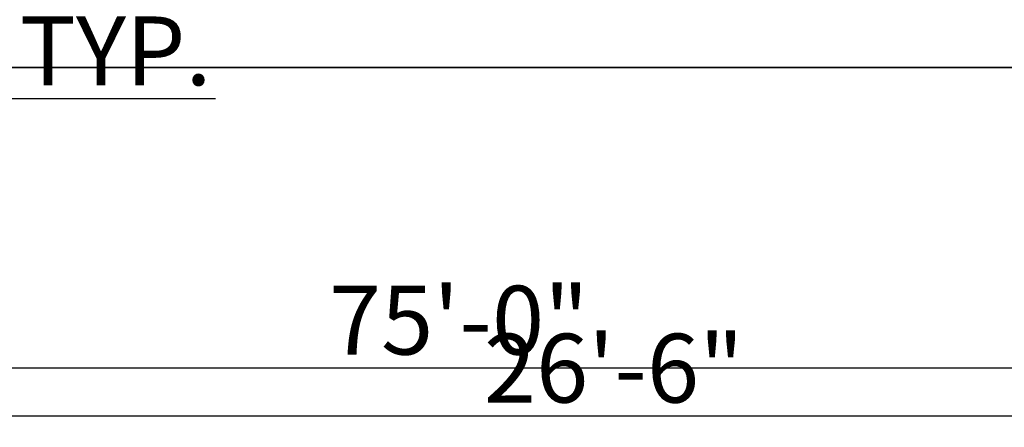
# Model space of a CAD drawing. Units: inches. Extents: x 2083 to 3317, y 1141 to 2115.
# Tile 106 of 256: x 2600 to 2772, y 1201 to 1272. Entities that reach past the tile are written whole.
import ezdxf

# ---------------------------------------------------------------- set-up
doc = ezdxf.new("R2010")
doc.units = ezdxf.units.IN
doc.layers.add('A-ANNO-DIMS', color=2, linetype='Continuous', lineweight=18)
doc.layers.add('A-WALL', color=7, linetype='Continuous', lineweight=35)
doc.layers.add('A-WALL-PATT', color=251, linetype='Continuous', lineweight=13, true_color=0x636466)
doc.styles.get("Standard").update_dxf_attribs({"font": 'arial.ttf'})
doc.dimstyles.new('ISO-25', dxfattribs={"dimtxt": 12, "dimasz": 12, "dimexe": 1.25, "dimexo": 0.625, "dimtad": 1, "dimlunit": 3, "dimtxsty": 'Standard', "dimcen": 2.5, "dimadec": 0, "dimazin": 0, "dimtfac": 1, "dimtmove": 0, "dimatfit": 3, "dimfxl": 1, "dimarcsym": 0})

# ---------------------------------------------------------------- blocks, each defined once
blk = doc.blocks.new('*D11')
at = {"layer": 'A-ANNO-DIMS', "color": 0, "lineweight": -2, "transparency": 16777216}
for p, q in [((2544.96, 1262.64), (2544.96, 1201.28)), ((2862.96, 1262.64), (2862.96, 1201.28)), ((2556.96, 1202.53), (2850.96, 1202.53))]:
    blk.add_line(p, q, dxfattribs=at)
at = {"layer": 'A-ANNO-DIMS', "color": 0, "transparency": 16777216}
for points in [[(2556.96, 1204.53), (2556.96, 1200.53), (2544.96, 1202.53)], [(2850.96, 1204.53), (2850.96, 1200.53), (2862.96, 1202.53)]]:
    blk.add_solid(points, dxfattribs=at)
at = {"layer": 'Defpoints', "color": 0, "transparency": 16777216}
for p in [(2544.96, 1263.26), (2862.96, 1263.26), (2862.96, 1202.53)]:
    blk.add_point(p, dxfattribs=at)
at = {"layer": 'A-ANNO-DIMS', "color": 0, "transparency": 16777216, "insert": (2703.96, 1209.29), "char_height": 12, "attachment_point": 5}
blk.add_mtext('26\'-6"', dxfattribs=at)
blk = doc.blocks.new('*D25')
at = {"layer": 'A-ANNO-DIMS', "color": 0, "lineweight": -2, "transparency": 16777216}
for p, q in [((2511.96, 1271.64), (2511.96, 1256.61)), ((2535.96, 1271.64), (2535.96, 1256.61)), ((2499.96, 1257.86), (2487.96, 1257.86)), ((2511.96, 1257.86), (2535.96, 1257.86)), ((2547.96, 1257.86), (2634.56, 1257.86))]:
    blk.add_line(p, q, dxfattribs=at)
at = {"layer": 'A-ANNO-DIMS', "color": 0, "transparency": 16777216}
for points in [[(2499.96, 1259.86), (2499.96, 1255.86), (2511.96, 1257.86)], [(2547.96, 1259.86), (2547.96, 1255.86), (2535.96, 1257.86)]]:
    blk.add_solid(points, dxfattribs=at)
at = {"layer": 'Defpoints', "color": 0, "transparency": 16777216}
for p in [(2511.96, 1272.26), (2535.96, 1272.26), (2535.96, 1257.86)]:
    blk.add_point(p, dxfattribs=at)
at = {"layer": 'A-ANNO-DIMS', "color": 0, "transparency": 16777216, "insert": (2597.26, 1264.61), "char_height": 12, "attachment_point": 5}
blk.add_mtext('2\'-0" TYP.', dxfattribs=at)
blk = doc.blocks.new('*D34')
at = {"layer": 'A-ANNO-DIMS', "color": 0, "lineweight": -2, "transparency": 16777216}
for p, q in [((2226.96, 1262.64), (2226.96, 1209.66)), ((3126.96, 1262.64), (3126.96, 1209.66)), ((2238.96, 1210.91), (3114.96, 1210.91))]:
    blk.add_line(p, q, dxfattribs=at)
at = {"layer": 'A-ANNO-DIMS', "color": 0, "transparency": 16777216}
for points in [[(2238.96, 1212.91), (2238.96, 1208.91), (2226.96, 1210.91)], [(3114.96, 1212.91), (3114.96, 1208.91), (3126.96, 1210.91)]]:
    blk.add_solid(points, dxfattribs=at)
at = {"layer": 'Defpoints', "color": 0, "transparency": 16777216}
for p in [(2226.96, 1263.26), (3126.96, 1263.26), (3126.96, 1210.91)]:
    blk.add_point(p, dxfattribs=at)
at = {"layer": 'A-ANNO-DIMS', "color": 0, "transparency": 16777216, "insert": (2676.96, 1217.66), "char_height": 12, "attachment_point": 5}
blk.add_mtext('75\'-0"', dxfattribs=at)

msp = doc.modelspace()

# ---------------------------------------------------------------- hatches: boundary and pattern name
at = {"layer": 'A-WALL-PATT'}
h = msp.add_hatch(color=256, dxfattribs=at)
h.dxf.hatch_style = 1
h.paths.add_polyline_path([(3126.96, 2020.761), (2748.96, 2020.761), (2604.96, 2020.761), (2226.96, 2020.761), (2226.96, 1702.761), (2466.96, 1702.761), (2466.96, 1582.761), (2418.96, 1582.761), (2418.96, 1477.761), (2226.96, 1477.761), (2226.96, 1263.261), (2544.96, 1263.261), (2544.96, 1411.761), (2604.96, 1411.761), (2685.96, 1411.761), (2685.96, 1420.761), (2604.96, 1420.761), (2604.96, 1573.761), (2604.96, 1702.761), (2604.96, 2011.761), (2748.96, 2011.761), (2748.96, 1702.761), (2862.96, 1702.761), (2862.96, 1621.761), (2871.96, 1621.761), (2871.96, 1702.761), (2883.96, 1702.761), (2883.96, 1706.939, -0.0264593), (2883.96, 1711.761), (2757.96, 1711.761), (2757.96, 1807.761), (2787.96, 1807.761), (2787.96, 1812.261), (2757.96, 1812.261), (2757.96, 2011.761), (2877.96, 2011.761), (2877.96, 1812.261), (2847.96, 1812.261), (2847.96, 1807.761), (2889.836, 1807.761), (2889.836, 1812.261), (2882.46, 1812.261), (2882.46, 2011.761), (3117.96, 2011.761), (3117.96, 1812.261), (2937.836, 1812.261), (2937.836, 1807.761), (2995.71, 1807.761), (2995.71, 1796.118), (3000.21, 1796.118), (3000.21, 1807.761), (3117.96, 1807.761), (3117.96, 1711.761), (3000.21, 1711.761), (3000.21, 1760.118), (2998.573, 1760.118, -0.020711), (2995.71, 1760.118), (2995.71, 1711.761), (2931.96, 1711.761), (2931.96, 1702.761), (3126.96, 1702.761)])
h.paths.add_polyline_path([(2471.46, 2011.761), (2471.46, 1810.011), (2462.717, 1810.011), (2462.717, 1805.511), (2505.96, 1805.511), (2505.96, 1810.011), (2475.96, 1810.011), (2475.96, 2011.761), (2595.96, 2011.761), (2595.96, 1810.011), (2565.96, 1810.011), (2565.96, 1805.511), (2595.96, 1805.511), (2595.96, 1711.761), (2235.96, 1711.761), (2235.96, 1805.511), (2353.71, 1805.511), (2353.71, 1796.054), (2358.21, 1796.054), (2358.21, 1805.511), (2414.717, 1805.511), (2414.717, 1810.011), (2235.96, 1810.011), (2235.96, 2011.761)], flags=16)
h.paths.add_polyline_path([(2270.205, 1994.61), (2270.205, 1970.61), (2246.205, 1970.61), (2246.205, 1994.61)], flags=0)
edge = h.paths.add_edge_path(flags=0)
edge.add_ellipse((2332.027, 1899.798), major_axis=(-3.043, 3.043), ratio=0.1682525, start_angle=-161.33217, end_angle=-156.30711, ccw=False)
edge.add_ellipse((2333.082, 1898.744), major_axis=(-1.055, 1.055), ratio=0.4535321, start_angle=-123.37102, end_angle=-94.15911)
edge = h.paths.add_edge_path(flags=0)
edge.add_ellipse((2332.027, 1968.876), major_axis=(3.043, 3.043), ratio=0.1682525, start_angle=18.66783, end_angle=23.69289)
edge.add_spline(control_points=[(2332.926, 1970.691), (2332.227, 1970.336), (2330.894, 1969.659), (2328.413, 1970.932), (2327.204, 1967.749), (2324.71, 1969.956), (2322.533, 1967.012), (2320.013, 1971.296), (2317.68, 1968.158), (2316.041, 1967.102), (2315.427, 1966.81)], knot_values=[0, 0, 0, 0, 2.2670587, 4.3245589, 6.6855835, 8.8786411, 11.121502, 14.300359, 17.7552837, 19.732645, 19.732645, 19.732645, 19.732645], degree=3, periodic=0)
edge.add_ellipse((2332.027, 1968.876), major_axis=(3.043, 3.043), ratio=0.1682525, start_angle=18.66783, end_angle=23.69289, ccw=False)
edge.add_ellipse((2333.082, 1969.931), major_axis=(1.055, 1.055), ratio=0.4535321, start_angle=56.62898, end_angle=85.84089, ccw=False)
edge = h.paths.add_edge_path(flags=0)
edge.add_spline(control_points=[(2296.428, 1967.988), (2293.628, 1965.336), (2287.704, 1959.727), (2299.744, 1949.996), (2294.533, 1935.669), (2290.573, 1920.604), (2293.394, 1909.974), (2296.185, 1904.967)], knot_values=[0.0991853, 0.0991853, 0.0991853, 0.0991853, 0.3453009, 0.6198217, 0.9826526, 1.3860932, 1.8105546, 1.8105546, 1.8105546, 1.8105546], degree=3, periodic=0)
edge.add_spline(control_points=[(2296.185, 1904.967), (2297.384, 1902.619), (2298.001, 1901.949), (2298.553, 1901.468)], knot_values=[0.0062457, 0.0062457, 0.0062457, 0.0062457, 0.0554759, 0.0554759, 0.0554759, 0.0554759], degree=3, periodic=0)
edge.add_spline(control_points=[(2298.553, 1901.468), (2297.259, 1900.923), (2295.225, 1900.232), (2293.06, 1900.614), (2292.101, 1900.788), (2292.09, 1900.791)], knot_values=[0.3128349, 0.3128349, 0.3128349, 0.3128349, 0.4017797, 0.4749867, 0.4759027, 0.4759027, 0.4759027, 0.4759027], degree=3, periodic=0)
edge.add_arc((2292.794, 1904.664), 3.937, 215.4209, 259.69818, ccw=False)
edge.add_spline(control_points=[(2289.585, 1902.382), (2289.477, 1902.535), (2289.368, 1902.688), (2289.261, 1902.841)], knot_values=[0.1028719, 0.1028719, 0.1028719, 0.1028719, 0.1168958, 0.1168958, 0.1168958, 0.1168958], degree=3, periodic=0)
edge.add_spline(control_points=[(2289.261, 1902.841), (2288.687, 1902.55), (2287.64, 1902.02), (2285.881, 1901.874), (2283.853, 1901.504), (2281.72, 1899.711), (2278.467, 1899.493), (2276.157, 1901.883), (2272.259, 1899.804), (2267.778, 1901.843), (2262.244, 1900.184), (2257.415, 1901.782), (2254.318, 1900.726), (2253.178, 1900.337)], knot_values=[0, 0, 0, 0, 1.9079767, 3.4771759, 5.261074, 7.9728515, 11.6802485, 13.7179214, 16.9395917, 22.789562, 27.5025027, 33.5952153, 37.1456181, 37.1456181, 37.1456181, 37.1456181], degree=3, periodic=0)
edge.add_line((2253.178, 1900.337), (2250.244, 1902.841))
edge.add_line((2250.244, 1902.841), (2250.244, 1965.833))
edge.add_line((2250.244, 1965.833), (2253.178, 1968.337))
edge.add_spline(control_points=[(2253.178, 1968.337), (2254.318, 1967.948), (2257.415, 1966.892), (2262.244, 1968.49), (2267.778, 1966.831), (2271.527, 1968.537), (2273.876, 1967.828), (2274.207, 1967.728)], knot_values=[0, 0, 0, 0, 0.0901802, 0.2449351, 0.3646438, 0.5132331, 0.5378548, 0.5378548, 0.5378548, 0.5378548], degree=3, periodic=0)
edge.add_arc((2274.353, 1963.793), 3.937, 72.05113, 92.12795, ccw=False)
edge.add_arc((2281.297, 1985.23), 18.596, 252.05113, 288.56572)
edge.add_arc((2292.317, 1956.029), 12.646, 71.02679, 113.77822, ccw=False)
edge = h.paths.add_edge_path(flags=0)
edge.add_spline(control_points=[(2274.899, 1951.856), (2275.066, 1951.617), (2275.233, 1951.377), (2275.398, 1951.136)], knot_values=[1.4099157, 1.4099157, 1.4099157, 1.4099157, 1.4315903, 1.4315903, 1.4315903, 1.4315903], degree=3, periodic=0)
edge.add_spline(control_points=[(2275.398, 1951.136), (2275.792, 1950.562), (2276.179, 1949.984), (2276.546, 1949.397)], knot_values=[1.3582378, 1.3582378, 1.3582378, 1.3582378, 1.4099157, 1.4099157, 1.4099157, 1.4099157], degree=3, periodic=0)
edge.add_line((2276.546, 1949.397), (2277.437, 1947.862))
edge.add_spline(control_points=[(2277.437, 1947.862), (2276.304, 1945.673), (2274.64, 1942.427), (2274.632, 1938.094), (2272.799, 1930.852), (2274.356, 1943.897), (2275.948, 1947.923), (2276.546, 1949.397)], knot_values=[0.0056315, 0.0056315, 0.0056315, 0.0056315, 0.1860139, 0.2660015, 0.3570872, 0.5963902, 0.7397317, 0.7397317, 0.7397317, 0.7397317], degree=3, periodic=0)
edge.add_spline(control_points=[(2276.546, 1949.397), (2276.179, 1949.984), (2275.792, 1950.562), (2275.398, 1951.136)], knot_values=[1.3582378, 1.3582378, 1.3582378, 1.3582378, 1.4099157, 1.4099157, 1.4099157, 1.4099157], degree=3, periodic=0)
edge.add_spline(control_points=[(2275.398, 1951.136), (2274.943, 1950.08), (2274.208, 1948.025), (2273.935, 1944.851), (2272.469, 1937.627), (2273.466, 1945.696), (2274.701, 1951.059), (2274.899, 1951.856)], knot_values=[0.1043639, 0.1043639, 0.1043639, 0.1043639, 0.1896363, 0.2696239, 0.3607096, 0.6000126, 0.6446217, 0.6446217, 0.6446217, 0.6446217], degree=3, periodic=0)
h.paths.add_polyline_path([(2269.168, 1963.128, -0.3575267), (2268.171, 1960.976, -0.0925607), (2268.171, 1939.436, -0.3575267), (2269.168, 1937.285, -0.3575267), (2267.016, 1938.282, -0.1647847), (2254.686, 1938.282, -0.3575267), (2252.534, 1937.285, -0.3575267), (2253.531, 1939.436, -0.0925607), (2253.531, 1960.976, -0.3575267), (2252.534, 1963.128, -0.3575267), (2254.686, 1962.131, -0.1647847), (2267.016, 1962.131, -0.3575267)], flags=0)
h.paths.add_polyline_path([(2248.874, 1967.802), (2248.874, 1957.028), (2249.458, 1957.028), (2249.458, 1911.647), (2248.874, 1911.647), (2248.874, 1900.873), (2246.512, 1900.873, 0.1973271), (2244.15, 1902.457), (2244.15, 1966.218, 0.1973271), (2246.512, 1967.802)], flags=0)
h.paths.add_polyline_path([(2269.168, 1931.389, -0.3575267), (2268.171, 1929.238, -0.0925607), (2268.171, 1907.698, -0.3575267), (2269.168, 1905.547, -0.3575267), (2267.016, 1906.544, -0.1647847), (2254.686, 1906.544, -0.3575267), (2252.534, 1905.547, -0.3575267), (2253.531, 1907.698, -0.0925607), (2253.531, 1929.238, -0.3575267), (2252.534, 1931.389, -0.3575267), (2254.686, 1930.392, -0.1647847), (2267.016, 1930.392, -0.3575267)], flags=0)
edge = h.paths.add_edge_path(flags=0)
edge.add_spline(control_points=[(2276.197, 1906.724), (2276.168, 1909.029), (2276.114, 1913.372), (2270.598, 1924.925), (2273.905, 1919.013), (2275.922, 1916.262), (2275.475, 1912.402), (2277.258, 1910.381), (2276.696, 1908.225), (2276.646, 1906.813), (2276.618, 1906.008)], knot_values=[0, 0, 0, 0, 8.6102597, 16.2212739, 18.8430575, 23.8048978, 27.4408283, 29.3561016, 31.2034776, 33.6506866, 33.6506866, 33.6506866, 33.6506866], degree=3, periodic=0)
edge.add_spline(control_points=[(2276.618, 1906.008), (2276.623, 1905.624), (2276.498, 1904.629), (2275.442, 1903.855), (2274.937, 1903.08), (2274.859, 1902.841)], knot_values=[0.1564884, 0.1564884, 0.1564884, 0.1564884, 0.1843975, 0.2313765, 0.2505985, 0.2505985, 0.2505985, 0.2505985], degree=3, periodic=0)
edge.add_line((2274.859, 1902.841), (2276.506, 1902.841))
edge.add_spline(control_points=[(2276.506, 1902.841), (2276.788, 1903.085), (2277.665, 1904.125), (2278.25, 1904.341), (2277.654, 1908.527), (2278.156, 1906.228), (2278.1, 1905.286), (2278.847, 1904.069), (2277.857, 1903.415), (2277.874, 1902.991), (2277.904, 1902.841)], knot_values=[0.0595743, 0.0595743, 0.0595743, 0.0595743, 0.0807529, 0.1037415, 0.1697201, 0.1760361, 0.2071372, 0.2404744, 0.2623409, 0.2736605, 0.2736605, 0.2736605, 0.2736605], degree=3, periodic=0)
edge.add_line((2277.904, 1902.841), (2280.03, 1902.841))
edge.add_spline(control_points=[(2280.03, 1902.841), (2279.888, 1903.088), (2279.499, 1903.982), (2280.152, 1905.939), (2278.104, 1909.658), (2279.762, 1907.185), (2280.328, 1904.875), (2280.485, 1903.49), (2281.463, 1903.249), (2281.758, 1902.936), (2281.834, 1902.841)], knot_values=[0.013856, 0.013856, 0.013856, 0.013856, 0.0348738, 0.0888667, 0.1078792, 0.1267378, 0.158714, 0.1937575, 0.2174868, 0.2267221, 0.2267221, 0.2267221, 0.2267221], degree=3, periodic=0)
edge.add_spline(control_points=[(2281.834, 1902.841), (2281.788, 1902.827), (2281.647, 1902.783), (2281.396, 1902.859), (2281.088, 1902.985), (2280.721, 1903.061), (2280.333, 1903.026), (2280.125, 1902.899), (2280.03, 1902.841)], knot_values=[0, 0, 0, 0, 0.1441304, 0.435517, 0.7492759, 1.1530457, 1.5483707, 1.878348, 1.878348, 1.878348, 1.878348], degree=3, periodic=0)
edge.add_line((2280.03, 1902.841), (2277.904, 1902.841))
edge.add_spline(control_points=[(2277.904, 1902.841), (2277.893, 1902.796), (2277.865, 1902.68), (2277.607, 1902.687), (2277.274, 1902.801), (2276.838, 1902.62), (2276.584, 1902.789), (2276.506, 1902.841)], knot_values=[0, 0, 0, 0, 0.1271885, 0.3261988, 0.6280094, 1.2435704, 1.5153306, 1.5153306, 1.5153306, 1.5153306], degree=3, periodic=0)
edge.add_line((2276.506, 1902.841), (2274.859, 1902.841))
edge.add_spline(control_points=[(2274.859, 1902.841), (2274.814, 1902.899), (2274.725, 1903.013), (2274.493, 1903.119), (2274.244, 1902.961), (2273.937, 1903.185), (2273.614, 1902.983), (2273.408, 1902.883), (2273.322, 1902.841)], knot_values=[0, 0, 0, 0, 0.2184302, 0.4369566, 0.6879766, 0.9903786, 1.3983955, 1.6918498, 1.6918498, 1.6918498, 1.6918498], degree=3, periodic=0)
edge.add_spline(control_points=[(2273.322, 1902.841), (2273.617, 1903.446), (2274.274, 1904.538), (2276.027, 1904.574), (2276.207, 1906.584), (2276.197, 1906.724)], knot_values=[0.0122268, 0.0122268, 0.0122268, 0.0122268, 0.0594721, 0.1062177, 0.134458, 0.134458, 0.134458, 0.134458], degree=3, periodic=0)
h.paths.add_polyline_path([(2270.776, 1897.79), (2270.776, 1873.79), (2246.776, 1873.79), (2246.776, 1897.79)], flags=0)
h.paths.add_polyline_path([(2353.71, 1760.005), (2353.71, 1760.054), (2358.21, 1760.054, -0.033729)], flags=0)
h.paths.add_polyline_path([(2321.819, 1737.529), (2341.995, 1737.529, -0.4142136), (2343.203, 1736.321), (2343.203, 1721.021, -0.4142136), (2341.995, 1719.813), (2321.819, 1719.813, -0.4142136), (2320.611, 1721.021), (2320.611, 1736.321, -0.4142136)], flags=0)
h.paths.add_polyline_path([(2324.235, 1736.321), (2339.579, 1736.321, -0.4142136), (2341.995, 1733.905), (2341.995, 1725.45, -0.4142136), (2339.579, 1723.034), (2333.681, 1723.034), (2333.845, 1722.045, -0.8706461), (2335.425, 1721.826, -0.767327), (2333.923, 1721.423), (2331.291, 1721.423, -0.767327), (2329.788, 1721.826, -0.8706461), (2331.368, 1722.045), (2331.533, 1723.034), (2324.235, 1723.034, -0.4142136), (2321.819, 1725.45), (2321.819, 1733.905, -0.4142136)], flags=0)
h.paths.add_polyline_path([(2570.484, 1928.615), (2589.684, 1928.615), (2590.169, 1928.615), (2590.169, 1904.993), (2570.484, 1904.993)], flags=0)
h.paths.add_polyline_path([(2574.447, 1927.264, -1), (2572.829, 1927.264, -1)], flags=0)
h.paths.add_polyline_path([(2573.09, 1926.941), (2573.925, 1927.776), (2574.148, 1927.553), (2573.313, 1926.718)], flags=0)
h.paths.add_polyline_path([(2578.779, 1919.73, -1), (2571.592, 1919.73, -1)], flags=0)
h.paths.add_polyline_path([(2578.385, 1919.73, -1), (2571.985, 1919.73, -1)], flags=0)
h.paths.add_polyline_path([(2331.596, 1729.476, -1), (2333.618, 1729.476, -1)], flags=0)
h.paths.add_polyline_path([(2578.034, 1927.264, -1), (2576.416, 1927.264, -1)], flags=0)
h.paths.add_polyline_path([(2576.689, 1927.531), (2576.912, 1927.754), (2577.747, 1926.919), (2577.524, 1926.696)], flags=0)
h.paths.add_polyline_path([(2578.139, 1909.86, -1), (2572.232, 1909.86, -1)], flags=0)
h.paths.add_polyline_path([(2577.745, 1909.86, -1), (2572.625, 1909.86, -1)], flags=0)
h.paths.add_polyline_path([(2583.798, 1927.264, -1), (2582.179, 1927.264, -1)], flags=0)
h.paths.add_polyline_path([(2582.719, 1927.754), (2583.554, 1926.919), (2583.331, 1926.696), (2582.496, 1927.531)], flags=0)
h.paths.add_polyline_path([(2582.496, 1927.531), (2582.719, 1927.754), (2583.554, 1926.919), (2583.331, 1926.696)], flags=0)
h.paths.add_polyline_path([(2587.739, 1920.53, -1), (2581.832, 1920.53, -1)], flags=0)
h.paths.add_polyline_path([(2587.345, 1920.53, -1), (2582.225, 1920.53, -1)], flags=0)
h.paths.add_polyline_path([(2587.385, 1927.264, -1), (2585.766, 1927.264, -1)], flags=0)
h.paths.add_polyline_path([(2586.082, 1926.98), (2586.917, 1927.815), (2587.14, 1927.593), (2586.305, 1926.758)], flags=0)
h.paths.add_polyline_path([(2588.379, 1910.66, -1), (2581.192, 1910.66, -1)], flags=0)
h.paths.add_polyline_path([(2587.985, 1910.66, -1), (2581.585, 1910.66, -1)], flags=0)
h.paths.add_polyline_path([(2417.168, 1729.478), (2437.344, 1729.478, -0.4142136), (2438.552, 1728.27), (2438.552, 1712.969, -0.4142136), (2437.344, 1711.761), (2417.168, 1711.761, -0.4142136), (2415.96, 1712.969), (2415.96, 1728.27, -0.4142136)], flags=0)
h.paths.add_polyline_path([(2419.584, 1728.27), (2434.928, 1728.27, -0.4142136), (2437.344, 1725.854), (2437.344, 1717.398, -0.4142136), (2434.928, 1714.983), (2429.029, 1714.983), (2429.194, 1713.994, -0.8706461), (2430.774, 1713.775, -0.767327), (2429.271, 1713.372), (2426.64, 1713.372, -0.767327), (2425.137, 1713.775, -0.8706461), (2426.717, 1713.994), (2426.882, 1714.983), (2419.584, 1714.983, -0.4142136), (2417.168, 1717.398), (2417.168, 1725.854, -0.4142136)], flags=0)
h.paths.add_polyline_path([(2419.584, 1728.27), (2434.928, 1728.27, -0.4142136), (2437.344, 1725.854), (2437.344, 1717.398, -0.4142136), (2434.928, 1714.983), (2429.029, 1714.983), (2428.358, 1719.009), (2427.553, 1719.009), (2426.882, 1714.983), (2419.584, 1714.983, -0.4142136), (2417.168, 1717.398), (2417.168, 1725.854, -0.4142136)], flags=0)
h.paths.add_polyline_path([(2426.944, 1721.425, -1), (2428.967, 1721.425, -1)], flags=0)
h.paths.add_polyline_path([(2475.96, 1702.761), (2595.96, 1702.761), (2595.96, 1582.761), (2475.96, 1582.761)], flags=16)
h.paths.add_polyline_path([(2427.96, 1573.761), (2595.96, 1573.761), (2595.96, 1468.761), (2595.96, 1420.761), (2384.46, 1420.761), (2384.46, 1468.761), (2427.96, 1468.761)], flags=16)
h.paths.add_polyline_path([(2379.96, 1468.761), (2379.96, 1420.761), (2235.96, 1420.761), (2235.96, 1468.761)], flags=16)
h.paths.add_polyline_path([(2317.816, 1466.696), (2337.992, 1466.696, -0.4142136), (2339.2, 1465.488), (2339.2, 1450.187, -0.4142136), (2337.992, 1448.979), (2317.816, 1448.979, -0.4142136), (2316.608, 1450.187), (2316.608, 1465.488, -0.4142136)], flags=0)
h.paths.add_polyline_path([(2320.232, 1465.488), (2335.576, 1465.488, -0.4142136), (2337.992, 1463.072), (2337.992, 1454.616, -0.4142136), (2335.576, 1452.2), (2329.677, 1452.2), (2329.842, 1451.212, -0.8706461), (2331.422, 1450.992, -0.767327), (2329.92, 1450.59), (2327.288, 1450.59, -0.767327), (2325.785, 1450.992, -0.8706461), (2327.365, 1451.212), (2327.53, 1452.2), (2320.232, 1452.2, -0.4142136), (2317.816, 1454.616), (2317.816, 1463.072, -0.4142136)], flags=0)
h.paths.add_polyline_path([(2320.232, 1465.488), (2335.576, 1465.488, -0.4142136), (2337.992, 1463.072), (2337.992, 1454.616, -0.4142136), (2335.576, 1452.2), (2329.677, 1452.2), (2329.006, 1456.227), (2328.201, 1456.227), (2327.53, 1452.2), (2320.232, 1452.2, -0.4142136), (2317.816, 1454.616), (2317.816, 1463.072, -0.4142136)], flags=0)
h.paths.add_polyline_path([(2327.593, 1458.643, -1), (2329.615, 1458.643, -1)], flags=0)
h.paths.add_polyline_path([(2244.412, 1433.34), (2241.921, 1433.34, -0.4142136), (2240.018, 1435.244), (2240.018, 1440.953, -0.4142105), (2241.921, 1442.856), (2244.412, 1442.856, -1.9764724)], flags=0)
h.paths.add_polyline_path([(2245.357, 1434.398, -0.4142136), (2245.357, 1441.799, -2.1440985)], flags=0)
h.paths.add_polyline_path([(2535.96, 1416.261), (2535.96, 1272.261), (2235.96, 1272.261), (2235.96, 1416.261)], flags=16)
h.paths.add_polyline_path([(2260.12, 1384.293), (2260.12, 1362.039), (2237.865, 1362.039), (2237.865, 1384.293)], flags=0)
edge = h.paths.add_edge_path(flags=0)
edge.add_line((2318.252, 1362.093), (2318.146, 1362.001))
edge.add_ellipse((2317.445, 1360.431), major_axis=(2.822, 2.822), ratio=0.1682525, start_angle=18.66783, end_angle=20.94813, ccw=False)
edge.add_ellipse((2318.423, 1361.409), major_axis=(0.978, 0.978), ratio=0.4535321, start_angle=56.62898, end_angle=70.2262, ccw=False)
edge = h.paths.add_edge_path(flags=0)
edge.add_line((2319.107, 1295.571), (2319.015, 1295.677))
edge.add_ellipse((2317.445, 1296.378), major_axis=(-2.822, 2.822), ratio=0.1682525, start_angle=-161.33217, end_angle=-159.05187, ccw=False)
edge.add_ellipse((2318.423, 1295.4), major_axis=(-0.978, 0.978), ratio=0.4535321, start_angle=-123.37102, end_angle=-109.7738)
edge = h.paths.add_edge_path(flags=0)
edge.add_spline(control_points=[(2284.21, 1301.17), (2284.581, 1300.445), (2284.891, 1299.892), (2285.16, 1299.461)], knot_values=[0.0390658, 0.0390658, 0.0390658, 0.0390658, 0.0554759, 0.0554759, 0.0554759, 0.0554759], degree=3, periodic=0)
edge.add_line((2285.16, 1299.461), (2284.21, 1301.17))
edge = h.paths.add_edge_path(flags=0)
edge.add_line((2280.412, 1297.298), (2283.37, 1297.036))
edge.add_line((2283.37, 1297.036), (2286.406, 1297.926))
edge.add_spline(control_points=[(2286.406, 1297.926), (2285.305, 1297.463), (2284.345, 1297.129), (2283.37, 1297.036)], knot_values=[0.3943688, 0.3943688, 0.3943688, 0.3943688, 0.4759027, 0.4759027, 0.4759027, 0.4759027], degree=3, periodic=0)
edge.add_spline(control_points=[(2283.37, 1297.036), (2283.281, 1297.028), (2282.316, 1296.957), (2281.313, 1297.134), (2280.423, 1297.296), (2280.412, 1297.298)], knot_values=[0.3128349, 0.3128349, 0.3128349, 0.3128349, 0.3202458, 0.3934528, 0.3943688, 0.3943688, 0.3943688, 0.3943688], degree=3, periodic=0)
edge = h.paths.add_edge_path(flags=0)
edge.add_line((2284.436, 1359.607), (2280.446, 1355.328))
edge.add_line((2280.446, 1355.328), (2279.58, 1351.018))
edge.add_line((2279.58, 1351.018), (2282.413, 1346.58))
edge.add_spline(control_points=[(2282.413, 1346.58), (2283.153, 1345.589), (2284.253, 1344.029), (2284.801, 1342.387), (2284.935, 1341.806)], knot_values=[1.2400982, 1.2400982, 1.2400982, 1.2400982, 1.3328922, 1.3827123, 1.3827123, 1.3827123, 1.3827123], degree=3, periodic=0)
edge.add_spline(control_points=[(2284.935, 1341.806), (2285.319, 1340.141), (2285.233, 1338.409), (2284.91, 1336.654)], knot_values=[1.0974841, 1.0974841, 1.0974841, 1.0974841, 1.2400982, 1.2400982, 1.2400982, 1.2400982], degree=3, periodic=0)
edge.add_spline(control_points=[(2284.91, 1336.654), (2284.587, 1334.899), (2284.027, 1333.12), (2283.463, 1331.361)], knot_values=[0.9548699, 0.9548699, 0.9548699, 0.9548699, 1.0974841, 1.0974841, 1.0974841, 1.0974841], degree=3, periodic=0)
edge.add_line((2283.463, 1331.361), (2281.89, 1326.153))
edge.add_line((2281.89, 1326.153), (2280.756, 1321.056))
edge.add_line((2280.756, 1321.056), (2280.299, 1316.002))
edge.add_line((2280.299, 1316.002), (2280.716, 1310.95))
edge.add_line((2280.716, 1310.95), (2282.028, 1305.972))
edge.add_line((2282.028, 1305.972), (2284.21, 1301.17))
edge.add_spline(control_points=[(2284.21, 1301.17), (2283.341, 1302.73), (2282.612, 1304.336), (2282.028, 1305.972)], knot_values=[0.0991853, 0.0991853, 0.0991853, 0.0991853, 0.2417994, 0.2417994, 0.2417994, 0.2417994], degree=3, periodic=0)
edge.add_spline(control_points=[(2282.028, 1305.972), (2281.444, 1307.608), (2281.005, 1309.273), (2280.716, 1310.95)], knot_values=[0.2417994, 0.2417994, 0.2417994, 0.2417994, 0.3844135, 0.3844135, 0.3844135, 0.3844135], degree=3, periodic=0)
edge.add_spline(control_points=[(2280.716, 1310.95), (2280.433, 1312.588), (2280.289, 1314.277), (2280.299, 1315.962), (2280.299, 1316.002)], knot_values=[0.3844135, 0.3844135, 0.3844135, 0.3844135, 0.5236467, 0.5270276, 0.5270276, 0.5270276, 0.5270276], degree=3, periodic=0)
edge.add_spline(control_points=[(2280.299, 1316.002), (2280.312, 1317.687), (2280.478, 1319.368), (2280.756, 1321.056)], knot_values=[0.5270276, 0.5270276, 0.5270276, 0.5270276, 0.6696417, 0.6696417, 0.6696417, 0.6696417], degree=3, periodic=0)
edge.add_spline(control_points=[(2280.756, 1321.056), (2281.035, 1322.744), (2281.426, 1324.44), (2281.89, 1326.153)], knot_values=[0.6696417, 0.6696417, 0.6696417, 0.6696417, 0.8122558, 0.8122558, 0.8122558, 0.8122558], degree=3, periodic=0)
edge.add_spline(control_points=[(2281.89, 1326.153), (2282.264, 1327.533), (2282.788, 1329.262), (2283.353, 1331.018), (2283.463, 1331.361)], knot_values=[0.8122558, 0.8122558, 0.8122558, 0.8122558, 0.9270873, 0.9548699, 0.9548699, 0.9548699, 0.9548699], degree=3, periodic=0)
edge.add_line((2283.463, 1331.361), (2284.91, 1336.654))
edge.add_line((2284.91, 1336.654), (2284.935, 1341.806))
edge.add_line((2284.935, 1341.806), (2282.413, 1346.58))
edge.add_spline(control_points=[(2282.413, 1346.58), (2281.275, 1348.104), (2280.078, 1349.57), (2279.58, 1351.018)], knot_values=[1.3827123, 1.3827123, 1.3827123, 1.3827123, 1.5253264, 1.5253264, 1.5253264, 1.5253264], degree=3, periodic=0)
edge.add_spline(control_points=[(2279.58, 1351.018), (2279.443, 1351.415), (2279.136, 1352.857), (2279.735, 1354.29), (2280.446, 1355.328)], knot_values=[1.5253264, 1.5253264, 1.5253264, 1.5253264, 1.564439, 1.6679405, 1.6679405, 1.6679405, 1.6679405], degree=3, periodic=0)
edge.add_spline(control_points=[(2280.446, 1355.328), (2281.426, 1356.758), (2282.931, 1358.183), (2284.436, 1359.607)], knot_values=[1.6679405, 1.6679405, 1.6679405, 1.6679405, 1.8105546, 1.8105546, 1.8105546, 1.8105546], degree=3, periodic=0)
edge.add_arc((2280.623, 1348.518), 11.726, 71.02679, 113.77822)
edge.add_arc((2270.405, 1375.595), 17.244, 252.05113, 288.56572, ccw=False)
edge.add_arc((2263.966, 1355.718), 3.651, 72.05113, 92.12795)
edge.add_arc((2263.966, 1355.718), 3.651, 92.12795, 177.98513)
edge.add_spline(control_points=[(2260.318, 1355.846), (2260.26, 1354.221), (2260.551, 1350.187), (2262.999, 1346.766), (2264.473, 1344.649)], knot_values=[1.4315903, 1.4315903, 1.4315903, 1.4315903, 1.5641438, 1.7706953, 1.7706953, 1.7706953, 1.7706953], degree=3, periodic=0)
edge.add_line((2264.473, 1344.649), (2264.936, 1343.983))
edge.add_spline(control_points=[(2263.801, 1340.248), (2263.843, 1340.514), (2264.067, 1341.756), (2264.513, 1343.002), (2264.935, 1343.981)], knot_values=[0.5365702, 0.5365702, 0.5365702, 0.5365702, 0.5593494, 0.6446217, 0.6446217, 0.6446217, 0.6446217], degree=3, periodic=0)
edge.add_spline(control_points=[(2264.935, 1343.981), (2265.118, 1343.715), (2265.299, 1343.448), (2265.477, 1343.179)], knot_values=[1.3840767, 1.3840767, 1.3840767, 1.3840767, 1.4099157, 1.4099157, 1.4099157, 1.4099157], degree=3, periodic=0)
edge.add_spline(control_points=[(2265.477, 1343.179), (2265.655, 1342.911), (2265.829, 1342.641), (2265.999, 1342.369)], knot_values=[1.3582378, 1.3582378, 1.3582378, 1.3582378, 1.3840767, 1.3840767, 1.3840767, 1.3840767], degree=3, periodic=0)
edge.add_line((2265.999, 1342.369), (2266.826, 1340.946))
edge.add_spline(control_points=[(2266.826, 1340.946), (2268.894, 1337.09), (2271.398, 1325.843), (2270.516, 1310.569), (2275.919, 1301.861), (2277.79, 1299.199)], knot_values=[0.1168958, 0.1168958, 0.1168958, 0.1168958, 0.4729873, 1.0509689, 1.3137934, 1.3137934, 1.3137934, 1.3137934], degree=3, periodic=0)
edge.add_spline(control_points=[(2277.79, 1299.199), (2277.839, 1299.128), (2277.889, 1299.057), (2277.94, 1298.987)], knot_values=[0.1098839, 0.1098839, 0.1098839, 0.1098839, 0.1168958, 0.1168958, 0.1168958, 0.1168958], degree=3, periodic=0)
edge.add_line((2277.94, 1298.987), (2277.789, 1299.199))
edge.add_spline(control_points=[(2277.789, 1299.199), (2277.257, 1298.929), (2276.286, 1298.438), (2275.039, 1298.334), (2274.383, 1298.239), (2274.215, 1298.209)], knot_values=[33.1218702, 33.1218702, 33.1218702, 33.1218702, 35.0290557, 36.5982549, 37.1448269, 37.1448269, 37.1448269, 37.1448269], degree=3, periodic=0)
edge.add_line((2274.215, 1298.209), (2273.073, 1297.893))
edge.add_spline(control_points=[(2273.073, 1297.893), (2272.323, 1297.58), (2271.039, 1296.511), (2269.248, 1296.226), (2268.423, 1296.375)], knot_values=[26.5325843, 26.5325843, 26.5325843, 26.5325843, 29.198919, 31.8391012, 31.8391012, 31.8391012, 31.8391012], degree=3, periodic=0)
edge.add_line((2268.423, 1296.375), (2263.879, 1297.458))
edge.add_spline(control_points=[(2263.879, 1297.458), (2263.556, 1297.359), (2261.86, 1296.839), (2260.239, 1297.282), (2258.933, 1297.516)], knot_values=[15.9195506, 15.9195506, 15.9195506, 15.9195506, 16.9395917, 21.2260675, 21.2260675, 21.2260675, 21.2260675], degree=3, periodic=0)
edge.add_line((2258.933, 1297.516), (2254.055, 1297.329))
edge.add_spline(control_points=[(2254.055, 1297.329), (2253.756, 1297.296), (2252.114, 1297.165), (2250.462, 1297.544), (2249.13, 1297.668)], knot_values=[5.3065169, 5.3065169, 5.3065169, 5.3065169, 6.2764352, 10.6130337, 10.6130337, 10.6130337, 10.6130337], degree=3, periodic=0)
edge.add_line((2249.13, 1297.668), (2244.332, 1296.878))
edge.add_line((2244.332, 1296.878), (2241.611, 1299.199))
edge.add_line((2241.611, 1299.199), (2241.611, 1357.609))
edge.add_line((2241.611, 1357.609), (2244.332, 1359.931))
edge.add_line((2244.332, 1359.931), (2252.729, 1359.543))
edge.add_spline(control_points=[(2252.729, 1359.543), (2252.871, 1359.546), (2253.306, 1359.548), (2253.74, 1359.514), (2254.032, 1359.482)], knot_values=[0.233291, 0.233291, 0.233291, 0.233291, 0.2449351, 0.2689274, 0.2689274, 0.2689274, 0.2689274], degree=3, periodic=0)
edge.add_line((2254.032, 1359.482), (2259.587, 1359.416))
edge.add_spline(control_points=[(2259.587, 1359.416), (2260.677, 1359.629), (2262.073, 1359.897), (2263.524, 1359.459), (2263.83, 1359.366)], knot_values=[0.4225164, 0.4225164, 0.4225164, 0.4225164, 0.5132331, 0.5378548, 0.5378548, 0.5378548, 0.5378548], degree=3, periodic=0)
edge.add_arc((2263.966, 1355.718), 3.651, 72.05113, 92.12795, ccw=False)
edge.add_arc((2270.405, 1375.595), 17.244, 252.05113, 288.56572)
edge.add_arc((2280.623, 1348.518), 11.726, 71.02679, 113.77822, ccw=False)
h.paths.add_polyline_path([(2240.341, 1359.435), (2240.341, 1349.444), (2240.882, 1349.444), (2240.882, 1307.365), (2240.341, 1307.365), (2240.341, 1297.374), (2238.15, 1297.374, 0.1973271), (2235.96, 1298.843), (2235.96, 1357.966, 0.1973271), (2238.15, 1359.435)], flags=0)
h.paths.add_polyline_path([(2259.158, 1355.101, -0.3575267), (2258.233, 1353.106, -0.0925607), (2258.233, 1333.133, -0.3575267), (2259.158, 1331.138, -0.3575267), (2257.163, 1332.062, -0.1647847), (2245.729, 1332.062, -0.3575267), (2243.735, 1331.138, -0.3575267), (2244.659, 1333.133, -0.0925607), (2244.659, 1353.106, -0.3575267), (2243.735, 1355.101, -0.3575267), (2245.729, 1354.176, -0.1647847), (2257.163, 1354.176, -0.3575267)], flags=0)
edge = h.paths.add_edge_path(flags=0)
edge.add_line((2265.999, 1342.369), (2266.826, 1340.946))
edge.add_line((2266.826, 1340.946), (2265.308, 1337.814))
edge.add_line((2265.308, 1337.814), (2264.358, 1334.653))
edge.add_line((2264.358, 1334.653), (2264.262, 1333.8))
edge.add_spline(control_points=[(2264.262, 1333.8), (2264.208, 1333.187), (2264.162, 1332.366), (2264.007, 1331.414), (2263.969, 1331.202)], knot_values=[0.4644442, 0.4644442, 0.4644442, 0.4644442, 0.5166905, 0.5316081, 0.5316081, 0.5316081, 0.5316081], degree=3, periodic=0)
edge.add_spline(control_points=[(2263.969, 1331.202), (2263.775, 1330.119), (2263.424, 1328.791), (2263.257, 1328.531), (2263.234, 1328.515)], knot_values=[0.3726816, 0.3726816, 0.3726816, 0.3726816, 0.4488497, 0.4644442, 0.4644442, 0.4644442, 0.4644442], degree=3, periodic=0)
edge.add_spline(control_points=[(2263.234, 1328.515), (2263.096, 1328.42), (2263.131, 1329.301), (2263.275, 1330.616)], knot_values=[0.2809191, 0.2809191, 0.2809191, 0.2809191, 0.3726816, 0.3726816, 0.3726816, 0.3726816], degree=3, periodic=0)
edge.add_spline(control_points=[(2263.275, 1330.616), (2263.419, 1331.93), (2263.672, 1333.677), (2263.97, 1335.315)], knot_values=[0.1891566, 0.1891566, 0.1891566, 0.1891566, 0.2809191, 0.2809191, 0.2809191, 0.2809191], degree=3, periodic=0)
edge.add_spline(control_points=[(2263.97, 1335.315), (2264.1, 1336.032), (2264.419, 1337.622), (2264.755, 1338.864), (2264.947, 1339.491)], knot_values=[0.097394, 0.097394, 0.097394, 0.097394, 0.1375775, 0.1891566, 0.1891566, 0.1891566, 0.1891566], degree=3, periodic=0)
edge.add_spline(control_points=[(2264.947, 1339.491), (2265.29, 1340.606), (2265.644, 1341.494), (2265.999, 1342.369)], knot_values=[0.0056315, 0.0056315, 0.0056315, 0.0056315, 0.097394, 0.097394, 0.097394, 0.097394], degree=3, periodic=0)
h.paths.add_polyline_path([(2259.158, 1325.671, -0.3575267), (2258.233, 1323.676, -0.0925607), (2258.233, 1303.703, -0.3575267), (2259.158, 1301.708, -0.3575267), (2257.163, 1302.633, -0.1647847), (2245.729, 1302.633, -0.3575267), (2243.735, 1301.708, -0.3575267), (2244.659, 1303.703, -0.0925607), (2244.659, 1323.676, -0.3575267), (2243.735, 1325.671, -0.3575267), (2245.729, 1324.747, -0.1647847), (2257.163, 1324.747, -0.3575267)], flags=0)
edge = h.paths.add_edge_path(flags=0)
edge.add_spline(control_points=[(2261.709, 1317.311), (2261.679, 1317.418), (2261.762, 1317.389), (2262.491, 1316.09), (2262.962, 1315.301)], knot_values=[14.9558607, 14.9558607, 14.9558607, 14.9558607, 16.2212739, 18.6948259, 18.6948259, 18.6948259, 18.6948259], degree=3, periodic=0)
edge.add_spline(control_points=[(2262.962, 1315.301), (2262.99, 1315.254), (2263.702, 1314.067), (2264.349, 1313.127), (2264.73, 1312.164)], knot_values=[18.6948259, 18.6948259, 18.6948259, 18.6948259, 18.8430575, 22.433791, 22.433791, 22.433791, 22.433791], degree=3, periodic=0)
edge.add_spline(control_points=[(2264.73, 1312.164), (2264.876, 1311.796), (2265.177, 1310.77), (2265.143, 1309.559), (2265.248, 1308.824)], knot_values=[22.433791, 22.433791, 22.433791, 22.433791, 23.8048978, 26.1727562, 26.1727562, 26.1727562, 26.1727562], degree=3, periodic=0)
edge.add_line((2265.248, 1308.824), (2265.851, 1307.172))
edge.add_spline(control_points=[(2265.851, 1307.172), (2266.065, 1306.822), (2266.384, 1306.332), (2266.424, 1305.781), (2266.42, 1305.611)], knot_values=[28.0625624, 28.0625624, 28.0625624, 28.0625624, 29.3561016, 29.9117214, 29.9117214, 29.9117214, 29.9117214], degree=3, periodic=0)
edge.add_spline(control_points=[(2266.42, 1305.611), (2266.416, 1305.433), (2266.394, 1305.25), (2266.365, 1305.066)], knot_values=[29.9117214, 29.9117214, 29.9117214, 29.9117214, 30.4978371, 30.4978371, 30.4978371, 30.4978371], degree=3, periodic=0)
edge.add_line((2266.365, 1305.066), (2266.066, 1302.136))
edge.add_spline(control_points=[(2266.066, 1302.136), (2266.071, 1301.78), (2265.998, 1301.2), (2265.663, 1300.759), (2265.509, 1300.586)], knot_values=[0.1564884, 0.1564884, 0.1564884, 0.1564884, 0.1843975, 0.2035434, 0.2035434, 0.2035434, 0.2035434], degree=3, periodic=0)
edge.add_line((2265.509, 1300.586), (2264.435, 1299.199))
edge.add_line((2264.435, 1299.199), (2265.962, 1299.199))
edge.add_line((2265.962, 1299.199), (2267.336, 1301.175))
edge.add_line((2267.336, 1301.175), (2267.312, 1301.986))
edge.add_spline(control_points=[(2267.312, 1301.986), (2267.261, 1302.862), (2267.16, 1303.737), (2267.271, 1303.326)], knot_values=[0.1262286, 0.1262286, 0.1262286, 0.1262286, 0.1666174, 0.1666174, 0.1666174, 0.1666174], degree=3, periodic=0)
edge.add_spline(control_points=[(2267.271, 1303.326), (2267.28, 1303.294), (2267.31, 1303.175), (2267.373, 1302.884), (2267.406, 1302.683), (2267.418, 1302.601)], knot_values=[0.1666174, 0.1666174, 0.1666174, 0.1666174, 0.1697201, 0.1760361, 0.1807647, 0.1807647, 0.1807647, 0.1807647], degree=3, periodic=0)
edge.add_spline(control_points=[(2267.744, 1300.988), (2267.688, 1301.151), (2267.481, 1301.657), (2267.484, 1302.145), (2267.418, 1302.601)], knot_values=[0.1807647, 0.1807647, 0.1807647, 0.1807647, 0.1937665, 0.2201389, 0.2201389, 0.2201389, 0.2201389], degree=3, periodic=0)
edge.add_line((2267.418, 1302.601), (2267.744, 1300.988))
edge.add_spline(control_points=[(2267.744, 1300.988), (2267.832, 1300.732), (2267.932, 1300.31), (2267.555, 1299.975), (2267.429, 1299.829)], knot_values=[0.2201389, 0.2201389, 0.2201389, 0.2201389, 0.2404744, 0.2548903, 0.2548903, 0.2548903, 0.2548903], degree=3, periodic=0)
edge.add_line((2267.429, 1299.829), (2267.258, 1299.199))
edge.add_line((2267.258, 1299.199), (2269.23, 1299.199))
edge.add_spline(control_points=[(2269.23, 1299.199), (2269.099, 1299.429), (2268.843, 1300.016), (2269.012, 1300.916), (2268.947, 1301.661)], knot_values=[0.013856, 0.013856, 0.013856, 0.013856, 0.0348738, 0.0670726, 0.0670726, 0.0670726, 0.0670726], degree=3, periodic=0)
edge.add_line((2268.947, 1301.661), (2268.432, 1303.603))
edge.add_spline(control_points=[(2268.432, 1303.603), (2268.176, 1304.192), (2267.596, 1305.251), (2268.041, 1304.623), (2268.251, 1304.282)], knot_values=[0.0901547, 0.0901547, 0.0901547, 0.0901547, 0.1078792, 0.1202891, 0.1202891, 0.1202891, 0.1202891], degree=3, periodic=0)
edge.add_spline(control_points=[(2268.251, 1304.282), (2268.361, 1304.105), (2269.058, 1302.918), (2269.383, 1301.59), (2269.521, 1300.776), (2269.575, 1300.556)], knot_values=[0.1202891, 0.1202891, 0.1202891, 0.1202891, 0.1267378, 0.158714, 0.1735056, 0.1735056, 0.1735056, 0.1735056], degree=3, periodic=0)
edge.add_line((2269.575, 1300.556), (2270.686, 1299.421))
edge.add_spline(control_points=[(2270.686, 1299.421), (2270.767, 1299.357), (2270.838, 1299.281), (2270.903, 1299.199)], knot_values=[0.2181597, 0.2181597, 0.2181597, 0.2181597, 0.2267221, 0.2267221, 0.2267221, 0.2267221], degree=3, periodic=0)
edge.add_line((2270.937, 1299.193), (2270.903, 1299.199))
edge.add_spline(control_points=[(2270.903, 1299.199), (2270.86, 1299.186), (2270.73, 1299.146), (2270.496, 1299.216), (2270.272, 1299.308), (2270.121, 1299.348), (2270.063, 1299.36)], knot_values=[0.939174, 0.939174, 0.939174, 0.939174, 1.0833044, 1.3746911, 1.6884499, 1.878348, 1.878348, 1.878348, 1.878348], degree=3, periodic=0)
edge.add_line((2270.063, 1299.36), (2269.23, 1299.199))
edge.add_line((2269.23, 1299.199), (2267.258, 1299.199))
edge.add_spline(control_points=[(2267.258, 1299.199), (2267.248, 1299.157), (2267.223, 1299.05), (2266.984, 1299.057), (2266.809, 1299.116), (2266.677, 1299.109), (2266.637, 1299.105)], knot_values=[0.7576653, 0.7576653, 0.7576653, 0.7576653, 0.8848538, 1.0838641, 1.3856747, 1.5153306, 1.5153306, 1.5153306, 1.5153306], degree=3, periodic=0)
edge.add_spline(control_points=[(2266.637, 1299.105), (2266.485, 1299.089), (2266.236, 1299.017), (2266.035, 1299.151), (2265.962, 1299.199)], knot_values=[0, 0, 0, 0, 0.4859051, 0.7576653, 0.7576653, 0.7576653, 0.7576653], degree=3, periodic=0)
edge.add_line((2265.962, 1299.199), (2264.435, 1299.199))
edge.add_line((2264.435, 1299.199), (2263.858, 1299.367))
edge.add_spline(control_points=[(2263.858, 1299.367), (2263.819, 1299.371), (2263.78, 1299.386), (2263.74, 1299.402)], knot_values=[0.8459249, 0.8459249, 0.8459249, 0.8459249, 0.9786272, 0.9786272, 0.9786272, 0.9786272], degree=3, periodic=0)
edge.add_line((2263.722, 1299.396), (2263.01, 1299.199))
edge.add_spline(control_points=[(2263.01, 1299.199), (2263.246, 1299.683), (2263.506, 1300.128), (2263.873, 1300.408)], knot_values=[0.0122268, 0.0122268, 0.0122268, 0.0122268, 0.0529705, 0.0529705, 0.0529705, 0.0529705], degree=3, periodic=0)
edge.add_spline(control_points=[(2263.873, 1300.408), (2263.932, 1300.453), (2264.084, 1300.553), (2264.255, 1300.624), (2264.36, 1300.665)], knot_values=[0.0529705, 0.0529705, 0.0529705, 0.0529705, 0.0594721, 0.0690861, 0.0690861, 0.0690861, 0.0690861], degree=3, periodic=0)
edge.add_line((2264.36, 1300.665), (2265.142, 1301.078))
edge.add_line((2265.142, 1301.078), (2265.676, 1302.8))
edge.add_line((2265.676, 1302.8), (2265.541, 1305.704))
edge.add_line((2265.541, 1305.704), (2264.803, 1309.328))
edge.add_line((2264.803, 1309.328), (2263.041, 1314.092))
edge.add_spline(control_points=[(2263.041, 1314.092), (2262.384, 1315.671), (2261.796, 1316.998), (2261.709, 1317.311)], knot_values=[11.2168955, 11.2168955, 11.2168955, 11.2168955, 14.9558607, 14.9558607, 14.9558607, 14.9558607], degree=3, periodic=0)
h.paths.add_polyline_path([(2871.96, 1416.261), (2895.91, 1416.261), (2895.91, 1420.761), (2871.96, 1420.761), (2871.96, 1501.761), (2862.96, 1501.761), (2862.96, 1420.761), (2805.96, 1420.761), (2805.96, 1411.761), (2862.96, 1411.761), (2862.96, 1263.261), (3126.96, 1263.261), (3126.96, 1411.761), (3126.96, 1486.761), (2943.96, 1486.761), (2943.96, 1477.761), (2967.86, 1477.761), (2967.86, 1420.761), (2943.91, 1420.761), (2943.91, 1416.261), (3117.96, 1416.261), (3117.96, 1420.761), (2972.36, 1420.761), (2972.36, 1477.761), (3117.96, 1477.761), (3117.96, 1420.761), (3117.96, 1272.261), (2871.96, 1272.261)], flags=0)
h.paths.add_polyline_path([(2457.126, 1485.943), (2527.603, 1485.943), (2527.603, 1537.636), (2457.126, 1537.636)], flags=8)
h.paths.add_polyline_path([(2481.005, 1609.982), (2590.766, 1609.982), (2590.766, 1682.003), (2481.005, 1682.003)], flags=8)
h.paths.add_polyline_path([(2483.085, 1729.127), (2553.562, 1729.127), (2553.562, 1780.82), (2483.085, 1780.82)], flags=8)

# ---------------------------------------------------------------- linework, layer by layer
at = {"layer": 'A-WALL'}
msp.add_line((2544.96, 1263.261), (3126.96, 1263.261), dxfattribs=at)

# ---------------------------------------------------------------- dimensions: what is measured, and where the dimension line sits
at = {"layer": 'A-ANNO-DIMS'}
dim = msp.add_linear_dim(base=(2535.96, 1257.861), p1=(2511.96, 1272.261), p2=(2535.96, 1272.261), text='<> TYP.', dimstyle='ISO-25', override={"dimdec": 1, "dimlfac": 1, "dimrnd": 0, "dimzin": 1, "dimdsep": 46, "dimlunit": 4, "dimfrac": 2}, dxfattribs=at)
dim.commit()
dim.dimension.update_dxf_attribs({"geometry": '*D25', "text_midpoint": (2597.26, 1264.613)})
for base, p1, p2, override, picture, middle in [((3126.96, 1210.911), (2226.96, 1263.261), (3126.96, 1263.261), {"dimdec": 1, "dimlfac": 1, "dimrnd": 0, "dimzin": 1, "dimdsep": 46, "dimlunit": 4, "dimfrac": 2}, '*D34', (2676.96, 1217.663)), ((2862.96, 1202.534), (2544.96, 1263.261), (2862.96, 1263.261), {"dimclrd": 0, "dimclre": 0, "dimclrt": 0}, '*D11', (2703.96, 1209.286))]:
    dim = msp.add_linear_dim(base=base, p1=p1, p2=p2, dimstyle='ISO-25', override=override, dxfattribs=at)
    dim.commit()
    dim.dimension.update_dxf_attribs({"geometry": picture, "text_midpoint": middle})

doc.saveas('drawing.dxf')
